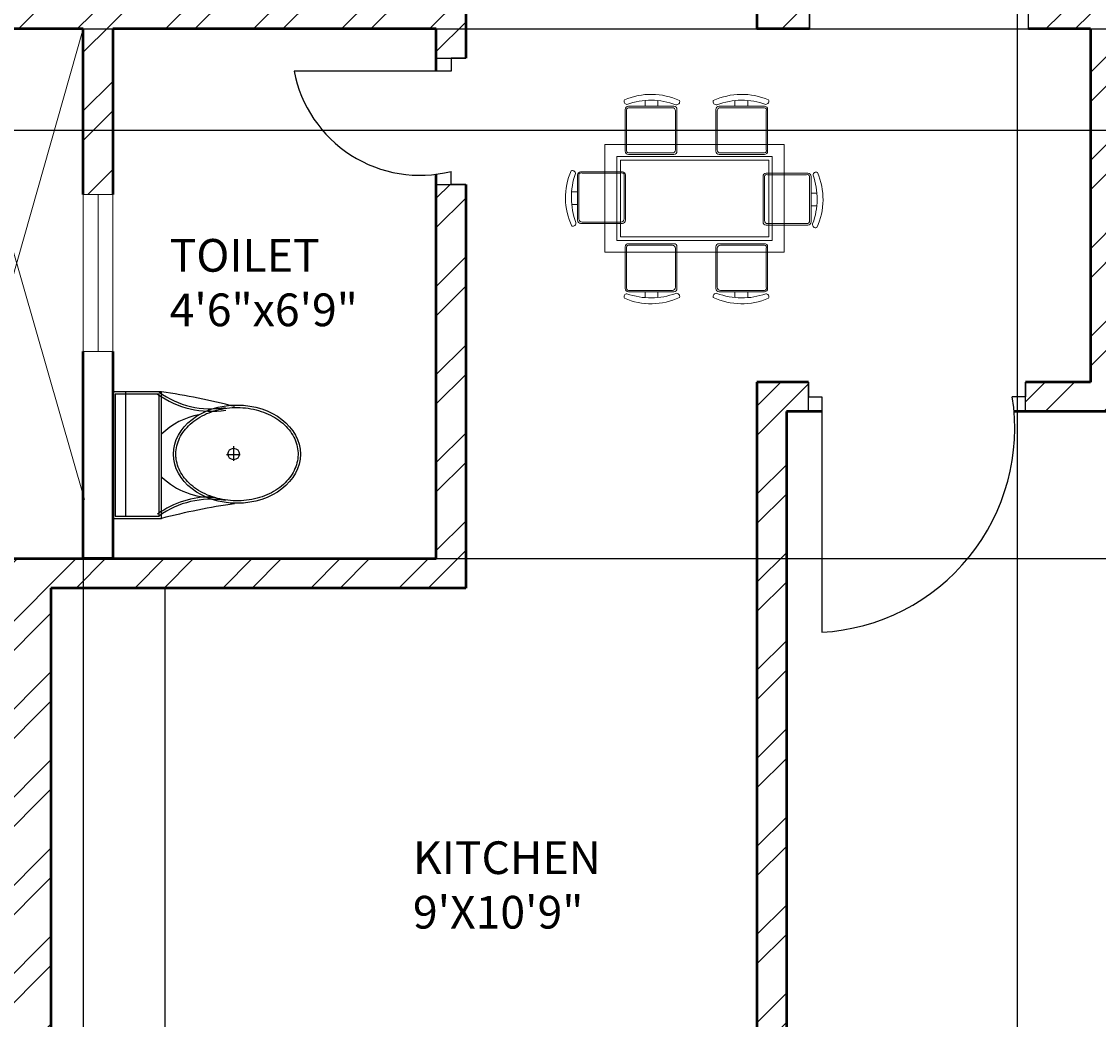
# Model space of a CAD drawing. Units: inches. Extents: x 1980 to 2738, y 1471 to 2568.
# Tile 12 of 22: x 2363 to 2528, y 1722 to 1874. Entities that reach past the tile are written whole.
import ezdxf

# ---------------------------------------------------------------- set-up
doc = ezdxf.new("R2010")
doc.units = ezdxf.units.IN
for name, color, linetype, lineweight in [('A-ANNO-DIMS', 2, 'Continuous', 18), ('A-AREA-IDEN', 7, 'Continuous', 18), ('A-DOOR', 31, 'Continuous', 25), ('A-FLOR-CASE', 8, 'Continuous', 25), ('A-FLOR-FIXT', 8, 'Continuous', 25), ('A-FLOR-OPEN', 8, 'Continuous', 18), ('A-FURN', 8, 'Continuous', 18), ('A-GLAZ', 141, 'Continuous', 18), ('A-WALL', 7, 'Continuous', 50)]:
    doc.layers.add(name, color=color, linetype=linetype, lineweight=lineweight)
doc.layers.add('A-WALL-PATT', color=9, linetype='Continuous', lineweight=13, true_color=0xd19cc7)
doc.styles.get("Standard").update_dxf_attribs({"font": 'arial.ttf'})
doc.dimstyles.get("Standard").update_dxf_attribs({"dimtxt": 0.18, "dimasz": 0.18, "dimexe": 0.18, "dimexo": 0.0625, "dimgap": 0.09, "dimtad": 0, "dimtih": 1, "dimtoh": 1, "dimdec": 4, "dimzin": 0, "dimdsep": 46, "dimtxsty": 'Standard', "dimcen": 0.09, "dimadec": 0, "dimazin": 0, "dimtfac": 1, "dimtdec": 4, "dimtofl": 0, "dimtmove": 0, "dimatfit": 3, "dimfxl": 1, "dimtolj": 1, "dimtzin": 0, "dimarcsym": 0})

# ---------------------------------------------------------------- blocks, each defined once
blk = doc.blocks.new('A$C31115884')
for p, q in [((283.1, 497.7), (223.4, 497.7)), ((257.5, 466.4), (257.5, 523.2)), ((0, 200), (0, 0)), ((520, 200), (0, 200)), ((10, 190), (10, 10)), ((510, 190), (10, 190)), ((510, 10), (510, 190)), ((520, 0), (520, 200)), ((510, 54.5), (0, 54.5)), ((10, 10), (510, 10)), ((0, 0), (520, 0))]:
    blk.add_line(p, q)
blk.add_circle((255.6, 496.4), 23.6)
for centre, radius, start, end in [((2777.7, -204.6), 2807, 165.4549, 171.7133), ((3237, 905), 2807, 188.2867, 194.5451), ((-294.5, 403.3), 364.7, 324.2091, 9.3499), ((-294.5, 403.3), 374.7, 324.2091, 9.3499), ((805.8, 403.3), 364.7, 170.6501, 215.7909), ((139.5, 406.2), 293.5, 315.8436, 2.6563), ((805.8, 403.3), 374.7, 179.2036, 215.7909), ((383.6, 406.2), 293.5, 190.2774, 224.1564)]:
    blk.add_arc(centre, radius, start, end)
blk.add_ellipse((256.2, 509.9), major_axis=(0, -260.7), ratio=0.772727)
blk.add_open_spline([(256.2, 259.2), (263.1, 259.2), (270, 259.7), (287.8, 262.3), (298.7, 265.1), (319.9, 273.1), (330.2, 278.4), (350.1, 291.1), (359.7, 298.7), (377.7, 315.9), (386.2, 325.5), (401.7, 346.6), (408.8, 358.1), (421.3, 382.5), (426.8, 395.5), (435.9, 422.4), (439.5, 436.4), (444.8, 465.1), (446.5, 479.7), (447.9, 509.2), (447.6, 524), (445, 553.3), (442.7, 567.8), (436.3, 596), (432.1, 609.7), (421.9, 636), (416, 648.6), (402.5, 672.1), (395, 683), (378.6, 703), (369.8, 712.1), (351.1, 728), (341.3, 734.8), (320.9, 746.2), (310.4, 750.7), (288.9, 757.3), (278, 759.4), (256, 761), (245, 760.6), (223.1, 757.2), (212.3, 754.3), (191.1, 746.1), (180.8, 740.7), (160.9, 727.8), (151.4, 720.1), (133.5, 702.7), (125.1, 693), (109.6, 671.7), (102.6, 660.2), (90.2, 635.7), (84.9, 622.7), (76, 595.6), (72.4, 581.6), (67.2, 552.9), (65.6, 538.2), (64.4, 508.8), (64.8, 494), (67.5, 464.7), (69.9, 450.2), (76.6, 422), (80.8, 408.3), (91.1, 382.2), (97.2, 369.7), (110.8, 346.3), (118.4, 335.4), (134.8, 315.6), (143.7, 306.7), (162.4, 290.9), (172.3, 284.2), (192.8, 273), (203.3, 268.6), (224.8, 262.2), (235.8, 260.2), (249.9, 259.3), (253, 259.2), (256.2, 259.2)], degree=3, knots=[0, 0, 0, 0, 0.110105, 0.110105, 0.285049, 0.285049, 0.459994, 0.459994, 0.634938, 0.634938, 0.809882, 0.809882, 0.984827, 0.984827, 1.159771, 1.159771, 1.334715, 1.334715, 1.50966, 1.50966, 1.684604, 1.684604, 1.859549, 1.859549, 2.034493, 2.034493, 2.209437, 2.209437, 2.384382, 2.384382, 2.559326, 2.559326, 2.73427, 2.73427, 2.909215, 2.909215, 3.084159, 3.084159, 3.259103, 3.259103, 3.434048, 3.434048, 3.608992, 3.608992, 3.783936, 3.783936, 3.958881, 3.958881, 4.133825, 4.133825, 4.30877, 4.30877, 4.483714, 4.483714, 4.658658, 4.658658, 4.833603, 4.833603, 5.008547, 5.008547, 5.183491, 5.183491, 5.358436, 5.358436, 5.53338, 5.53338, 5.708324, 5.708324, 5.883269, 5.883269, 6.058213, 6.058213, 6.233158, 6.233158, 6.283185, 6.283185, 6.283185, 6.283185])
blk = doc.blocks.new('TABLE-DINING-RECT')
for points in [[(0, 16.47), (27.45, 16.47), (27.45, 0), (0, 0)], [(0, 16.47), (27.45, 16.47), (27.45, 0), (0, 0)], [(1.83, 14.64), (25.62, 14.64), (25.62, 1.83), (1.83, 1.83)], [(1.83, 14.64), (25.62, 14.64), (25.62, 1.83), (1.83, 1.83)], [(2.38, 14.09), (25.07, 14.09), (25.07, 2.38), (2.38, 2.38)], [(2.38, 14.09), (25.07, 14.09), (25.07, 2.38), (2.38, 2.38)]]:
    blk.add_lwpolyline(points, close=True)
blk = doc.blocks.new('WIN-24IN-PARTITION')
for p, q in [((0, 24), (4.5, 24)), ((0, 24), (0, 0)), ((4.5, 24), (2.25, 24)), ((2.25, 24), (2.25, 0)), ((4.5, 24), (4.5, 0)), ((2.25, 0), (0, 0)), ((0, 0), (4.5, 0))]:
    blk.add_line(p, q)
blk = doc.blocks.new('SHAFT-OPENING-MARK')
for p, q in [((20.51, 72), (0, 0)), ((0, 72), (20.71, 0.06))]:
    blk.add_line(p, q)
blk = doc.blocks.new('*D41')
at = {"layer": 'A-ANNO-DIMS', "color": 0, "lineweight": -2, "transparency": 16777216}
for p, q in [((2298.65, 2095.14), (2298.65, 1533.71)), ((2515.4, 2095.14), (2515.4, 1533.71)), ((2298.83, 1533.89), (2406.56, 1533.89)), ((2515.22, 1533.89), (2407.49, 1533.89))]:
    blk.add_line(p, q, dxfattribs=at)
at = {"layer": 'A-ANNO-DIMS', "color": 0, "transparency": 16777216}
for points in [[(2298.83, 1533.92), (2298.83, 1533.86), (2298.65, 1533.89)], [(2515.22, 1533.92), (2515.22, 1533.86), (2515.4, 1533.89)]]:
    blk.add_solid(points, dxfattribs=at)
at = {"layer": 'Defpoints', "color": 0, "transparency": 16777216}
for p in [(2298.65, 2095.21), (2515.4, 2095.21), (2515.4, 1533.89)]:
    blk.add_point(p, dxfattribs=at)
at = {"layer": 'A-ANNO-DIMS', "color": 0, "transparency": 16777216, "insert": (2407.03, 1533.89), "char_height": 0.18, "attachment_point": 5}
blk.add_mtext('\\A1;216.75', dxfattribs=at)
blk = doc.blocks.new('*D57')
at = {"layer": 'A-ANNO-DIMS', "color": 0, "lineweight": -2, "transparency": 16777216}
for p, q in [((2351.81, 1792.14), (2351.81, 1533.71)), ((2372.53, 1792.14), (2372.53, 1533.71)), ((2351.99, 1533.89), (2361.77, 1533.89)), ((2372.35, 1533.89), (2362.56, 1533.89))]:
    blk.add_line(p, q, dxfattribs=at)
at = {"layer": 'A-ANNO-DIMS', "color": 0, "transparency": 16777216}
for points in [[(2351.99, 1533.92), (2351.99, 1533.86), (2351.81, 1533.89)], [(2372.35, 1533.92), (2372.35, 1533.86), (2372.53, 1533.89)]]:
    blk.add_solid(points, dxfattribs=at)
at = {"layer": 'Defpoints', "color": 0, "transparency": 16777216}
for p in [(2351.81, 1792.21), (2372.53, 1792.21), (2372.53, 1533.89)]:
    blk.add_point(p, dxfattribs=at)
at = {"layer": 'A-ANNO-DIMS', "color": 0, "transparency": 16777216, "insert": (2362.17, 1533.89), "char_height": 0.18, "attachment_point": 5}
blk.add_mtext('\\A1;20.72', dxfattribs=at)
blk = doc.blocks.new('*D58')
at = {"layer": 'A-ANNO-DIMS', "color": 0, "lineweight": -2, "transparency": 16777216}
for p, q in [((2372.59, 1873.21), (2689.91, 1873.21)), ((2689.73, 1873.03), (2689.73, 1832.89)), ((2689.73, 1792.39), (2689.73, 1832.52)), ((2372.59, 1792.21), (2689.91, 1792.21))]:
    blk.add_line(p, q, dxfattribs=at)
at = {"layer": 'A-ANNO-DIMS', "color": 0, "transparency": 16777216}
for points in [[(2689.7, 1873.03), (2689.76, 1873.03), (2689.73, 1873.21)], [(2689.7, 1792.39), (2689.76, 1792.39), (2689.73, 1792.21)]]:
    blk.add_solid(points, dxfattribs=at)
at = {"layer": 'Defpoints', "color": 0, "transparency": 16777216}
for p in [(2372.53, 1873.21), (2689.73, 1873.21), (2372.53, 1792.21)]:
    blk.add_point(p, dxfattribs=at)
at = {"layer": 'A-ANNO-DIMS', "color": 0, "transparency": 16777216, "insert": (2689.73, 1832.71), "char_height": 0.18, "attachment_point": 5}
blk.add_mtext('\\A1;81', dxfattribs=at)
blk = doc.blocks.new('*D61')
at = {"layer": 'A-ANNO-DIMS', "color": 0, "lineweight": -2, "transparency": 16777216}
for p, q in [((2114.15, 1873.21), (2689.91, 1873.21)), ((2689.73, 1873.03), (2689.73, 1865.65)), ((2689.73, 1857.91), (2689.73, 1865.29)), ((2114.15, 1857.73), (2689.91, 1857.73))]:
    blk.add_line(p, q, dxfattribs=at)
at = {"layer": 'A-ANNO-DIMS', "color": 0, "transparency": 16777216}
for points in [[(2689.7, 1873.03), (2689.76, 1873.03), (2689.73, 1873.21)], [(2689.7, 1857.91), (2689.76, 1857.91), (2689.73, 1857.73)]]:
    blk.add_solid(points, dxfattribs=at)
at = {"layer": 'Defpoints', "color": 0, "transparency": 16777216}
for p in [(2114.08, 1873.21), (2689.73, 1873.21), (2114.08, 1857.73)]:
    blk.add_point(p, dxfattribs=at)
at = {"layer": 'A-ANNO-DIMS', "color": 0, "transparency": 16777216, "insert": (2689.73, 1865.47), "char_height": 0.18, "attachment_point": 5}
blk.add_mtext('\\A1;15.48', dxfattribs=at)

msp = doc.modelspace()

# ---------------------------------------------------------------- hatches: boundary and pattern name
at = {"layer": 'A-WALL-PATT'}
h = msp.add_hatch(dxfattribs=at)
h.set_pattern_fill('ANSI32', color=256)
h.paths.add_polyline_path([(2257.5661, 2416.2064), (2257.5661, 2420.7064), (2250.5833, 2420.7064), (2250.5833, 2462.7064), (2246.0833, 2462.7064), (2246.0833, 2420.7064), (2237.0791, 2420.7064), (2237.0791, 2411.7064), (2246.0833, 2411.7064), (2246.0833, 2291.7064), (2242.6109, 2291.7064), (2242.6109, 2287.2064), (2246.0833, 2287.2064), (2250.5833, 2287.2064), (2250.5833, 2291.7064), (2250.5833, 2411.7064), (2257.5661, 2411.7064)])
h.paths.add_polyline_path([(2387.0396, 2416.2064), (2387.0396, 2420.7064), (2367.5833, 2420.7064), (2367.5833, 2462.7064), (2358.5833, 2462.7064), (2358.5833, 2420.7064), (2329.3087, 2420.7064), (2329.3087, 2411.7064), (2358.5833, 2411.7064), (2358.5833, 2321.7275), (2358.5833, 2309.7064), (2347.3089, 2309.7064), (2293.3089, 2309.7064), (2293.3089, 2259.0771), (2297.8089, 2259.0771), (2297.8089, 2305.2064), (2347.3089, 2305.2064), (2347.3089, 2284.7412), (2351.8089, 2284.7412), (2351.8089, 2305.2064), (2372.3188, 2305.2064), (2372.3761, 2284.3899), (2377.0295, 2284.3899), (2377.0295, 2299.3058), (2377.0295, 2305.2064), (2426.5295, 2305.2064), (2426.5295, 2257.5573), (2431.0295, 2257.5573), (2431.0295, 2309.7064), (2377.0295, 2309.7064), (2367.5833, 2309.7064), (2367.5833, 2321.7275), (2367.5833, 2411.7064), (2387.0396, 2411.7064)])
h.paths.add_polyline_path([(2448.5267, 2416.2064), (2448.5267, 2420.7064), (2423.0396, 2420.7064), (2423.0396, 2411.7064), (2448.5267, 2411.7064)])
h.paths.add_polyline_path([(2130.9128, 2416.2064), (2130.9128, 2420.7064), (2105.0833, 2420.7064), (2105.0833, 2386.6942), (2114.0833, 2386.6942), (2114.0833, 2411.7064), (2130.9128, 2411.7064)])
h.paths.add_polyline_path([(2212.9478, 2420.7064), (2190.9128, 2420.7064), (2190.9128, 2411.7064), (2212.9478, 2411.7064), (2212.9478, 2416.2064)])
h.paths.add_polyline_path([(2114.0833, 2326.6942), (2105.0833, 2326.6942), (2105.0833, 2291.7064), (2081.0833, 2291.7064), (2081.0833, 2287.2064), (2105.0833, 2287.2064), (2105.0833, 2276.1935), (2114.0833, 2276.1935), (2114.0833, 2287.2064), (2166.3825, 2287.2064), (2166.3825, 2289.4564), (2166.3825, 2291.7064), (2114.0833, 2291.7064)])
h.paths.add_polyline_path([(2114.0833, 2252.1935), (2105.0833, 2252.1935), (2105.0833, 2233.2064), (2081.0833, 2233.2064), (2081.0833, 2228.7064), (2105.0833, 2228.7064), (2105.0833, 2213.4478), (2114.0833, 2213.4478), (2114.0833, 2228.7064), (2195.0833, 2228.7064), (2199.5833, 2228.7064), (2208.4455, 2228.7064), (2208.4455, 2230.9564), (2208.4455, 2233.2064), (2199.5833, 2233.2064), (2199.5833, 2287.2064), (2206.8904, 2287.2064), (2206.8904, 2289.4564), (2206.8904, 2291.7064), (2189.446, 2291.7064), (2189.446, 2289.4564), (2189.446, 2287.2064), (2195.0833, 2287.2064), (2195.0833, 2233.2064), (2114.0833, 2233.2064)])
h.paths.add_polyline_path([(2114.0833, 2153.4478), (2109.5833, 2153.4478), (2105.0833, 2153.4478), (2105.0833, 2135.2374), (2114.0833, 2135.2374)], flags=17)
h.paths.add_polyline_path([(2135.9619, 2095.4081), (2140.1805, 2095.4081), (2140.1805, 2104.2064), (2114.0833, 2104.2064), (2114.0833, 2110.3997), (2109.5833, 2110.3997), (2105.0833, 2110.3997), (2105.0833, 2104.2064), (2081.0833, 2104.2064), (2081.0833, 2099.7064), (2105.0833, 2099.7064), (2127.5416, 2099.8532), (2127.5416, 2056.9393), (2136.2133, 2056.9393)], flags=17)
h.paths.add_polyline_path([(2255.4895, 2104.2064), (2250.5833, 2104.2064), (2250.5833, 2233.2064), (2246.0833, 2233.2064), (2242.4941, 2233.2064), (2242.4941, 2228.7064), (2246.0833, 2228.7064), (2246.0833, 2104.2064), (2163.6825, 2104.2064), (2163.6825, 2099.8072), (2163.6825, 2095.4081), (2191.4325, 2095.4081), (2191.4325, 2011.2064), (2186.0833, 2011.2064), (2136.5143, 2010.8824), (2136.3702, 2032.9403), (2131.9559, 2032.9115), (2127.5416, 2032.8826), (2127.5416, 2006.7064), (2105.0833, 2006.7064), (2081.0833, 2006.7064), (2081.0833, 2002.2064), (2105.0833, 2002.2064), (2105.0833, 1995.9329), (2114.0833, 1995.9329), (2114.0833, 2002.2064), (2246.0833, 2002.2064), (2246.0833, 1877.7064), (2242.1358, 1877.7064), (2242.1358, 1873.2064), (2250.5833, 1873.2064), (2250.5833, 2002.2064), (2255.3335, 2002.2064), (2255.3335, 2011.2064), (2195.9325, 2011.2064), (2195.9325, 2095.2064), (2255.4895, 2095.2064), (2255.4895, 2099.5471)])
h.paths.add_polyline_path([(2199.5833, 1873.2064), (2209.827, 1873.2064), (2209.827, 1875.4564), (2209.827, 1877.7064), (2114.0833, 1877.7064), (2114.0833, 1890.0968), (2105.0833, 1890.0968), (2105.0833, 1877.7064), (2081.0833, 1877.7064), (2081.0833, 1873.2064), (2105.0833, 1873.2064), (2105.0833, 1857.7279), (2114.0833, 1857.7279), (2114.0833, 1873.2064), (2195.0833, 1873.2064), (2195.0833, 1819.2064), (2190.298, 1819.2064), (2190.298, 1814.7064), (2209.8976, 1814.7064), (2209.8976, 1816.9564), (2209.8976, 1819.2064), (2199.5833, 1819.2064)])
h.paths.add_polyline_path([(2114.0833, 1814.7064), (2166.2538, 1814.7064), (2166.2538, 1816.9564), (2166.2538, 1819.2064), (2114.0833, 1819.2064), (2114.0833, 1833.7279), (2109.5833, 1833.7279), (2105.0833, 1833.7279), (2105.0833, 1819.2064), (2081.0833, 1819.2064), (2081.0833, 1814.7064), (2105.0833, 1814.7064), (2105.0833, 1782.5516), (2114.0833, 1782.5516)])
h.paths.add_polyline_path([(2114.0833, 1722.5516), (2109.5833, 1722.5516), (2105.0833, 1722.5516), (2105.0833, 1685.7064), (2124.5104, 1685.7064), (2124.5104, 1690.2064), (2124.5104, 1694.7064), (2114.0833, 1694.7064)])
h.paths.add_polyline_path([(2218.8787, 1694.7064), (2184.5104, 1694.7064), (2184.5104, 1685.7064), (2218.8787, 1685.7064), (2218.8787, 1690.2064)])
h.paths.add_polyline_path([(2250.5833, 1819.2064), (2242.6431, 1819.2064), (2242.6431, 1816.9564), (2242.6431, 1814.7064), (2246.0833, 1814.7064), (2246.0833, 1694.7064), (2240.4035, 1694.7064), (2240.4035, 1690.2064), (2240.4035, 1685.7064), (2246.0833, 1685.7064), (2246.0833, 1643.7064), (2250.5833, 1643.7064), (2250.5833, 1685.7064), (2255.9859, 1685.7064), (2255.9859, 1690.2064), (2255.9859, 1694.7064), (2250.5833, 1694.7064)])
h.paths.add_polyline_path([(2297.4764, 1694.7064), (2279.3934, 1694.7064), (2279.3934, 1690.2064), (2279.3934, 1685.7064), (2297.4764, 1685.7064), (2297.4764, 1690.2064)])
h.paths.add_polyline_path([(2377.1596, 1694.7064), (2367.5833, 1694.7064), (2367.5833, 1787.7064), (2431.0295, 1787.7064), (2431.0295, 1792.2064), (2431.0295, 1849.4149), (2428.7795, 1849.4149), (2426.5295, 1849.4149), (2426.5295, 1792.2064), (2421.5833, 1792.2064), (2367.5833, 1792.2064), (2297.8089, 1792.2064), (2297.8089, 1850.2946), (2295.5589, 1850.2946), (2293.3089, 1850.2946), (2293.3089, 1792.2064), (2293.3089, 1787.7064), (2297.8089, 1787.7064), (2358.5833, 1787.7064), (2358.5833, 1694.7064), (2333.4764, 1694.7064), (2333.4764, 1685.7064), (2358.5833, 1685.7064), (2358.5833, 1643.7064), (2367.5833, 1643.7064), (2367.5833, 1685.7064), (2377.1596, 1685.7064)])
h.paths.add_polyline_path([(2442.4912, 1694.7064), (2413.1596, 1694.7064), (2413.1596, 1685.7064), (2442.4912, 1685.7064)])
h.paths.add_polyline_path([(2480.0833, 1814.7064), (2483.4816, 1814.7064), (2483.4816, 1817.9384), (2483.4816, 1819.2064), (2475.5833, 1819.2064), (2475.5833, 1694.7064), (2470.7283, 1694.7064), (2470.7283, 1685.7064), (2475.5833, 1685.7064), (2475.5833, 1643.7064), (2480.0833, 1643.7064), (2480.0833, 1685.7064), (2486.3293, 1685.7064), (2486.3293, 1690.2064), (2486.3293, 1694.7064), (2480.0833, 1694.7064)])
h.paths.add_polyline_path([(2621.0833, 1721.7349), (2612.0833, 1721.7349), (2612.0833, 1694.7064), (2586.1453, 1694.7064), (2586.1453, 1685.7064), (2621.0833, 1685.7064)])
h.paths.add_polyline_path([(2526.1453, 1690.2064), (2526.1453, 1694.7064), (2511.584, 1694.7064), (2511.584, 1690.2064), (2511.584, 1685.7064), (2526.1453, 1685.7064)])
h.paths.add_polyline_path([(2645.0833, 1819.2064), (2621.0833, 1819.2064), (2621.0833, 1835.8527), (2616.5833, 1835.8527), (2612.0833, 1835.8527), (2612.0833, 1819.2064), (2560.2541, 1819.2064), (2560.2541, 1814.7064), (2612.0833, 1814.7064), (2612.0833, 1781.7349), (2621.0833, 1781.7349), (2621.0833, 1814.7064), (2645.0833, 1814.7064)])
h.paths.add_polyline_path([(2645.0833, 1877.7064), (2621.0833, 1877.7064), (2621.0833, 1886.4375), (2612.0833, 1886.4375), (2612.0833, 1877.7064), (2517.1032, 1877.7064), (2517.1032, 1875.4564), (2517.1032, 1873.2064), (2526.5833, 1873.2064), (2526.5833, 1819.2064), (2516.6454, 1819.2064), (2516.6454, 1816.9564), (2516.6454, 1814.7064), (2536.4445, 1814.7064), (2536.4445, 1816.9564), (2536.4445, 1819.2064), (2531.0833, 1819.2064), (2531.0833, 1873.2064), (2612.0833, 1873.2064), (2612.0833, 1859.8527), (2621.0833, 1859.8527), (2621.0833, 1873.2064), (2645.0833, 1873.2064)])
h.paths.add_polyline_path([(2645.0833, 2006.7064), (2621.0833, 2006.7064), (2588.5085, 2006.7064), (2588.5085, 2052.9125), (2579.9045, 2052.9125), (2579.9045, 2011.2064), (2519.9045, 2011.2064), (2519.9045, 2095.2064), (2553.1204, 2095.2064), (2553.1204, 2104.2064), (2480.0833, 2104.2064), (2480.0833, 2228.7064), (2484.3832, 2228.7064), (2484.3832, 2230.9564), (2484.3832, 2233.2064), (2475.5833, 2233.2064), (2475.5833, 2104.2064), (2463.1308, 2104.2064), (2463.1308, 2095.2064), (2501.2463, 2095.2064), (2510.9045, 2095.2064), (2515.4045, 2095.2064), (2515.4045, 2011.2064), (2510.9045, 2011.2064), (2501.2463, 2011.2064), (2462.5957, 2011.2064), (2462.5957, 2002.2064), (2475.5833, 2002.2064), (2475.5833, 1873.2064), (2483.6146, 1873.2064), (2483.6146, 1875.4564), (2483.6146, 1877.7064), (2480.0833, 1877.7064), (2480.0833, 2002.2064), (2612.0833, 2002.2064), (2612.0833, 1996.309), (2621.0833, 1996.309), (2621.0833, 2002.2064), (2645.0833, 2002.2064)])
h.paths.add_polyline_path([(2588.5085, 2099.7277), (2621.0833, 2099.7277), (2645.0833, 2099.7064), (2645.0833, 2104.2064), (2621.0833, 2104.2064), (2621.0833, 2109.0038), (2616.5833, 2109.0038), (2612.0833, 2109.0038), (2612.0833, 2104.2064), (2575.0621, 2104.2064), (2575.0621, 2099.7064), (2575.0621, 2095.2064), (2579.9045, 2095.2064), (2579.9045, 2076.9125), (2588.5085, 2076.9125)], flags=17)
h.paths.add_polyline_path([(2367.5833, 2002.2064), (2373.7228, 2002.2064), (2373.7228, 2006.7064), (2373.7228, 2011.2064), (2350.7889, 2011.2064), (2350.7889, 2006.7064), (2350.7889, 2002.2064), (2358.5833, 2002.2064), (2358.5833, 1877.7064), (2293.3089, 1877.7064), (2293.3089, 1870.4987), (2297.8089, 1870.4987), (2297.8089, 1873.2064), (2347.3089, 1873.2064), (2347.3089, 1847.2208), (2351.8089, 1847.2208), (2351.8089, 1873.2064), (2372.5295, 1873.2064), (2372.5295, 1847.8619), (2377.0295, 1847.8619), (2377.0295, 1873.2064), (2426.5295, 1873.2064), (2426.5295, 1868.7339), (2431.0295, 1868.7339), (2431.0295, 1877.7064), (2367.5833, 1877.7064)])
h.paths.add_polyline_path([(2531.0833, 2287.2064), (2534.2285, 2287.2064), (2534.2285, 2291.7064), (2516.7886, 2291.7064), (2516.7886, 2287.2064), (2526.5833, 2287.2064), (2526.5833, 2233.2064), (2517.9112, 2233.2064), (2517.9112, 2230.9564), (2517.9112, 2228.7064), (2526.5833, 2228.7064), (2531.0833, 2228.7064), (2612.0833, 2228.7064), (2612.0833, 2206.8504), (2621.0833, 2206.8504), (2621.0833, 2228.7064), (2645.0833, 2228.7064), (2645.0833, 2233.2064), (2621.0833, 2233.2064), (2621.0833, 2241.8536), (2616.5833, 2241.8536), (2612.0833, 2241.8536), (2612.0833, 2233.2064), (2531.0833, 2233.2064)])
h.paths.add_polyline_path([(2645.0833, 2291.7064), (2621.0833, 2291.7064), (2621.0833, 2323.0138), (2616.5833, 2323.0138), (2612.0833, 2323.0138), (2612.0833, 2291.7064), (2559.6852, 2291.7064), (2559.6852, 2289.4564), (2559.6852, 2287.2064), (2612.0833, 2287.2064), (2612.0833, 2265.8536), (2621.0833, 2265.8536), (2621.0833, 2287.2064), (2645.0833, 2287.2064)])
h.paths.add_polyline_path([(2621.0833, 2420.7064), (2582.8189, 2420.7064), (2582.8189, 2411.7064), (2612.0833, 2411.7064), (2612.0833, 2383.0138), (2621.0833, 2383.0138)])
h.paths.add_polyline_path([(2480.0833, 2411.7064), (2485.7342, 2411.7064), (2485.7342, 2416.2064), (2485.7342, 2420.7064), (2480.0833, 2420.7064), (2480.0833, 2462.7064), (2475.5833, 2462.7064), (2475.5833, 2420.7064), (2469.4083, 2420.7064), (2469.4083, 2411.7064), (2475.5833, 2411.7064), (2475.5833, 2291.7064), (2475.5833, 2287.2064), (2482.9195, 2287.2064), (2482.9195, 2289.4564), (2482.9195, 2291.7064), (2480.0833, 2291.7064)])
h.paths.add_polyline_path([(2367.5833, 2228.7064), (2431.0295, 2228.7064), (2431.0295, 2233.2064), (2431.0295, 2237.4203), (2428.7795, 2237.4203), (2426.5295, 2237.4203), (2426.5295, 2233.2064), (2377.0295, 2233.2064), (2377.0295, 2260.3837), (2372.4423, 2260.3837), (2372.517, 2233.2635), (2351.8089, 2233.2064), (2351.8089, 2260.7412), (2347.3089, 2260.7412), (2347.3089, 2233.2064), (2297.8089, 2233.2064), (2297.8089, 2236.9324), (2293.3089, 2236.9324), (2293.3089, 2228.7064), (2358.5833, 2228.7064), (2358.5833, 2104.2064), (2353.3665, 2104.2064), (2353.3665, 2095.2064), (2373.8869, 2095.2064), (2373.8869, 2099.7064), (2373.8869, 2104.2064), (2367.5833, 2104.2064)])
h.paths.add_polyline_path([(2321.2323, 2104.2064), (2303.4895, 2104.2064), (2303.4895, 2095.2064), (2321.2323, 2095.2064), (2321.2323, 2099.7064)], flags=0)
h.paths.add_polyline_path([(2415.1308, 2099.7064), (2415.1308, 2104.2064), (2404.81, 2104.2064), (2404.81, 2095.2064), (2415.1308, 2095.2064)], flags=17)
h.paths.add_polyline_path([(2318.6336, 2011.2064), (2303.3335, 2011.2064), (2303.3335, 2002.2064), (2318.6336, 2002.2064)], flags=0)
h.paths.add_polyline_path([(2414.5957, 2011.2064), (2406.2461, 2011.2064), (2406.2461, 2006.7064), (2406.2461, 2002.2064), (2414.5957, 2002.2064)], flags=17)

# ---------------------------------------------------------------- linework, layer by layer
at = {"layer": 'A-DOOR'}
for p, q in [((2483.6146, 1877.7064), (2483.6146, 1873.2064)), ((2517.1032, 1873.2064), (2517.1032, 1877.7064)), ((2483.6146, 1873.2064), (2483.6146, 1875.4564)), ((2426.5295, 1868.7339), (2431.0295, 1868.7339)), ((2431.0295, 1868.7339), (2428.7795, 1868.7339)), ((2428.7795, 1868.7339), (2428.7795, 1868.7339)), ((2428.7795, 1868.7339), (2428.7795, 1866.7339)), ((2428.7795, 1866.7339), (2404.7795, 1866.7339)), ((2428.7795, 1849.4149), (2428.7795, 1851.4149)), ((2426.5295, 1849.4149), (2431.0295, 1849.4149)), ((2431.0295, 1849.4149), (2428.7795, 1849.4149)), ((2483.4816, 1817.9384), (2483.4816, 1819.2064)), ((2483.4816, 1819.2064), (2483.4816, 1816.9444)), ((2516.6454, 1814.7064), (2516.6454, 1819.2064)), ((2516.6454, 1819.2064), (2516.6454, 1816.9564)), ((2483.4816, 1814.7064), (2483.4816, 1817.9384)), ((2483.4816, 1816.9444), (2485.4816, 1816.9444)), ((2485.4816, 1816.9444), (2485.4816, 1780.9444)), ((2516.6454, 1816.9564), (2514.6454, 1816.9564))]:
    msp.add_line(p, q, dxfattribs=at)
for centre, radius, start, end in [((2424.0189, 1870.4161), 19.5886, 190.83485, 284.065556), ((2483.7368, 1812.1723), 31.2767, 273.198076, 8.798569)]:
    msp.add_arc(centre, radius, start, end, dxfattribs=at)
at = {"layer": 'A-FLOR-CASE'}
msp.add_line((2384.9917, 1787.7064), (2384.9917, 1711.1804), dxfattribs=at)
at = {"layer": 'A-FURN'}
for points in [[(2455.6982, 1861.6711, -0.17580919), (2463.1736, 1861.6144, 0.57839206), (2463.7399, 1862.2372, 0.21452438), (2455.3018, 1862.3504, 0.55201397), (2455.6982, 1861.6711, -0.06507904)], [(2455.6982, 1861.6708, -0.17580919), (2463.1736, 1861.6142, 0.57839206), (2463.74, 1862.2369, 0.21452438), (2455.3018, 1862.3501, 0.55201397), (2455.6982, 1861.6708, -0.06507904)], [(2469.467, 1861.6144, -0.57839206), (2468.9006, 1862.2372, -0.21452438), (2477.3388, 1862.3504, -0.55201397), (2476.9424, 1861.6711, 0.1758092), (2469.467, 1861.6144)], [(2469.467, 1861.6142, -0.57839206), (2468.9007, 1862.2369, -0.21452438), (2477.3388, 1862.3501, -0.55201397), (2476.9424, 1861.6708, 0.1758092), (2469.467, 1861.6142)], [(2460.4188, 1861.371), (2460.4188, 1862.2487, -0.06475861)], [(2460.4188, 1861.3707), (2460.4188, 1862.2484, -0.06475861)], [(2472.2218, 1861.371), (2472.2218, 1862.2487, 0.06475861)], [(2472.2218, 1861.3707), (2472.2218, 1862.2484, 0.06475861)], [(2462.8565, 1861.371), (2455.9165, 1861.371, 0.41421356), (2455.431, 1860.8855), (2455.431, 1854.5044, 0.41421356), (2455.9165, 1854.0188), (2462.8565, 1854.0188, 0.41421356), (2463.342, 1854.5044), (2463.342, 1860.8855, 0.41421356), (2462.8565, 1861.371)], [(2462.8565, 1861.3707), (2455.9165, 1861.3707, 0.41421356), (2455.431, 1860.8852), (2455.431, 1854.5041, 0.41421356), (2455.9165, 1854.0185), (2462.8565, 1854.0185, 0.41421356), (2463.342, 1854.5041), (2463.342, 1860.8852, 0.41421356), (2462.8565, 1861.3707)], [(2476.7241, 1861.371, -0.41421356), (2477.2096, 1860.8855), (2477.2096, 1854.5044, -0.41421356), (2476.7241, 1854.0188), (2469.7841, 1854.0188, -0.41421356), (2469.2986, 1854.5044), (2469.2986, 1860.8855, -0.41421356), (2469.7841, 1861.371), (2476.7241, 1861.371)], [(2476.7241, 1861.3707, -0.41421356), (2477.2096, 1860.8852), (2477.2096, 1854.5041, -0.41421356), (2476.7241, 1854.0185), (2469.7841, 1854.0185, -0.41421356), (2469.2986, 1854.5041), (2469.2986, 1860.8852, -0.41421356), (2469.7841, 1861.3707), (2476.7241, 1861.3707)], [(2447.8774, 1843.619, -0.57839206), (2447.2547, 1843.0527, -0.21452438), (2447.1415, 1851.4909, -0.55201397), (2447.8208, 1851.0944, 0.17580937), (2447.8774, 1843.619)], [(2447.8775, 1843.6187, -0.57839206), (2447.2547, 1843.0524, -0.21452438), (2447.1415, 1851.4906, -0.55201397), (2447.8208, 1851.0942, 0.17580937), (2447.8775, 1843.6187)], [(2448.1209, 1850.8761, -0.41421356), (2448.6064, 1851.3616), (2454.9875, 1851.3616, -0.41421356), (2455.4731, 1850.8761), (2455.4731, 1843.9362, -0.41421356), (2454.9875, 1843.4506), (2448.6064, 1843.4506, -0.41421356), (2448.1209, 1843.9362), (2448.1209, 1850.8761)], [(2448.1209, 1850.8758, -0.41421356), (2448.6064, 1851.3613), (2454.9875, 1851.3613, -0.41421356), (2455.4731, 1850.8758), (2455.4731, 1843.9359, -0.41421356), (2454.9875, 1843.4503), (2448.6064, 1843.4503, -0.41421356), (2448.1209, 1843.9359), (2448.1209, 1850.8758)], [(2483.8583, 1850.6384, 0.41421356), (2483.3728, 1851.1239), (2476.9916, 1851.1239, 0.41421356), (2476.5061, 1850.6384), (2476.5061, 1843.6985, 0.41421356), (2476.9916, 1843.213), (2483.3728, 1843.213, 0.41421356), (2483.8583, 1843.6985), (2483.8583, 1850.6384)], [(2483.8583, 1850.6381, 0.41421356), (2483.3728, 1851.1237), (2476.9917, 1851.1237, 0.41421356), (2476.5061, 1850.6381), (2476.5061, 1843.6982, 0.41421356), (2476.9917, 1843.2127), (2483.3728, 1843.2127, 0.41421356), (2483.8583, 1843.6982), (2483.8583, 1850.6381)], [(2484.1583, 1850.8568, -0.17580919), (2484.1017, 1843.3813, 0.57839206), (2484.7244, 1842.815, 0.21452438), (2484.8377, 1851.2532, 0.55201397), (2484.1583, 1850.8568, -0.06507904)], [(2484.1584, 1850.8565, -0.17580919), (2484.1018, 1843.381, 0.57839206), (2484.7245, 1842.8147, 0.21452438), (2484.8377, 1851.2529, 0.55201397), (2484.1584, 1850.8565, -0.06507904)], [(2448.1209, 1846.3738), (2447.2432, 1846.3738, 0.06475861)], [(2448.1209, 1846.3735), (2447.2432, 1846.3735, 0.06475861)], [(2483.8583, 1846.1361), (2484.736, 1846.1361, -0.06475861)], [(2483.8583, 1846.1358), (2484.736, 1846.1358, -0.06475861)], [(2462.8565, 1833.0053), (2455.9165, 1833.0053, -0.41421356), (2455.431, 1833.4908), (2455.431, 1839.8719, -0.41421356), (2455.9165, 1840.3575), (2462.8565, 1840.3575, -0.41421356), (2463.342, 1839.8719), (2463.342, 1833.4908, -0.41421356), (2462.8565, 1833.0053)], [(2462.8565, 1833.005), (2455.9165, 1833.005, -0.41421356), (2455.431, 1833.4905), (2455.431, 1839.8717, -0.41421356), (2455.9165, 1840.3572), (2462.8565, 1840.3572, -0.41421356), (2463.342, 1839.8717), (2463.342, 1833.4905, -0.41421356), (2462.8565, 1833.005)], [(2476.7241, 1833.0053, 0.41421356), (2477.2096, 1833.4908), (2477.2096, 1839.8719, 0.41421356), (2476.7241, 1840.3575), (2469.7841, 1840.3575, 0.41421356), (2469.2986, 1839.8719), (2469.2986, 1833.4908, 0.41421356), (2469.7841, 1833.0053), (2476.7241, 1833.0053)], [(2476.7241, 1833.005, 0.41421356), (2477.2096, 1833.4905), (2477.2096, 1839.8717, 0.41421356), (2476.7241, 1840.3572), (2469.7841, 1840.3572, 0.41421356), (2469.2986, 1839.8717), (2469.2986, 1833.4905, 0.41421356), (2469.7841, 1833.005), (2476.7241, 1833.005)], [(2463.1736, 1832.7619, -0.57839206), (2463.7399, 1832.1391, -0.21452438), (2455.3018, 1832.0259, -0.55201397), (2455.6982, 1832.7052, 0.17580929), (2463.1736, 1832.7619)], [(2463.1736, 1832.7616, -0.57839206), (2463.74, 1832.1389, -0.21452438), (2455.3018, 1832.0256, -0.55201397), (2455.6982, 1832.705, 0.17580929), (2463.1736, 1832.7616)], [(2460.4188, 1833.0053), (2460.4188, 1832.1276, 0.06475861)], [(2460.4188, 1833.005), (2460.4188, 1832.1273, 0.06475861)], [(2476.9424, 1832.7052, -0.17580928), (2469.467, 1832.7619, 0.57839206), (2468.9006, 1832.1391, 0.21452438), (2477.3388, 1832.0259, 0.55201397), (2476.9424, 1832.7052, -0.06507904)], [(2476.9424, 1832.705, -0.17580928), (2469.467, 1832.7616, 0.57839206), (2468.9007, 1832.1389, 0.21452438), (2477.3388, 1832.0256, 0.55201397), (2476.9424, 1832.705, -0.06507904)], [(2472.2218, 1833.0053), (2472.2218, 1832.1276, -0.06475861)], [(2472.2218, 1833.005), (2472.2218, 1832.1273, -0.06475861)]]:
    msp.add_lwpolyline(points, format="xyb", dxfattribs=at)
for points in [[(2458.4762, 1862.2647), (2458.4762, 1861.371)], [(2458.4762, 1862.2644), (2458.4762, 1861.3707)], [(2474.1644, 1862.2647), (2474.1644, 1861.371)], [(2474.1644, 1862.2644), (2474.1644, 1861.3707)], [(2447.2272, 1848.3164), (2448.1209, 1848.3164)], [(2447.2272, 1848.3161), (2448.1209, 1848.3161)], [(2484.752, 1848.0787), (2483.8583, 1848.0787)], [(2484.752, 1848.0784), (2483.8583, 1848.0784)], [(2458.4762, 1832.1116), (2458.4762, 1833.0053)], [(2458.4762, 1832.1113), (2458.4762, 1833.005)], [(2474.1644, 1832.1116), (2474.1644, 1833.0053)], [(2474.1644, 1832.1113), (2474.1644, 1833.005)]]:
    msp.add_lwpolyline(points, dxfattribs=at)
for points in [[(2455.9195, 1861.1523), (2462.6377, 1861.1523, -0.41421356), (2463.1233, 1860.6668), (2463.1233, 1854.7231, -0.41421356), (2462.6377, 1854.2376), (2455.9195, 1854.2376, -0.51206948), (2455.6497, 1854.7231), (2455.6497, 1860.6668, -0.51206948)], [(2455.9195, 1861.152), (2462.6377, 1861.152, -0.41421356), (2463.1233, 1860.6665), (2463.1233, 1854.7228, -0.41421356), (2462.6377, 1854.2373), (2455.9195, 1854.2373, -0.51206948), (2455.6497, 1854.7228), (2455.6497, 1860.6665, -0.51206948)], [(2476.7211, 1861.1523), (2470.0029, 1861.1523, 0.41421356), (2469.5173, 1860.6668), (2469.5173, 1854.7231, 0.41421356), (2470.0029, 1854.2376), (2476.7211, 1854.2376, 0.51206948), (2476.9909, 1854.7231), (2476.9909, 1860.6668, 0.51206948)], [(2476.7211, 1861.152), (2470.0029, 1861.152, 0.41421356), (2469.5173, 1860.6665), (2469.5173, 1854.7228, 0.41421356), (2470.0029, 1854.2373), (2476.7211, 1854.2373, 0.51206948), (2476.9909, 1854.7228), (2476.9909, 1860.6665, 0.51206948)], [(2448.3396, 1850.8732), (2448.3396, 1844.1549, 0.41421356), (2448.8251, 1843.6694), (2454.7688, 1843.6694, 0.41421356), (2455.2543, 1844.1549), (2455.2543, 1850.8732, 0.51206948), (2454.7688, 1851.1429), (2448.8251, 1851.1429, 0.51206948)], [(2448.3396, 1850.8729), (2448.3396, 1844.1546, 0.41421356), (2448.8251, 1843.6691), (2454.7688, 1843.6691, 0.41421356), (2455.2543, 1844.1546), (2455.2543, 1850.8729, 0.51206948), (2454.7688, 1851.1426), (2448.8251, 1851.1426, 0.51206948)], [(2483.6396, 1850.6355), (2483.6396, 1843.9172, -0.41421356), (2483.1541, 1843.4317), (2477.2104, 1843.4317, -0.41421356), (2476.7249, 1843.9172), (2476.7249, 1850.6355, -0.51206948), (2477.2104, 1850.9052), (2483.1541, 1850.9052, -0.51206948)], [(2483.6396, 1850.6352), (2483.6396, 1843.9169, -0.41421356), (2483.1541, 1843.4314), (2477.2104, 1843.4314, -0.41421356), (2476.7249, 1843.9169), (2476.7249, 1850.6352, -0.51206948), (2477.2104, 1850.9049), (2483.1541, 1850.9049, -0.51206948)], [(2455.9195, 1833.224), (2462.6377, 1833.224, 0.41421356), (2463.1233, 1833.7095), (2463.1233, 1839.6532, 0.41421356), (2462.6377, 1840.1387), (2455.9195, 1840.1387, 0.51206948), (2455.6497, 1839.6532), (2455.6497, 1833.7095, 0.51206948)], [(2455.9195, 1833.2237), (2462.6377, 1833.2237, 0.41421356), (2463.1233, 1833.7092), (2463.1233, 1839.6529, 0.41421356), (2462.6377, 1840.1385), (2455.9195, 1840.1385, 0.51206948), (2455.6497, 1839.6529), (2455.6497, 1833.7092, 0.51206948)], [(2476.7211, 1833.224), (2470.0029, 1833.224, -0.41421356), (2469.5173, 1833.7095), (2469.5173, 1839.6532, -0.41421356), (2470.0029, 1840.1387), (2476.7211, 1840.1387, -0.51206948), (2476.9909, 1839.6532), (2476.9909, 1833.7095, -0.51206948)], [(2476.7211, 1833.2237), (2470.0029, 1833.2237, -0.41421356), (2469.5173, 1833.7092), (2469.5173, 1839.6529, -0.41421356), (2470.0029, 1840.1385), (2476.7211, 1840.1385, -0.51206948), (2476.9909, 1839.6529), (2476.9909, 1833.7092, -0.51206948)]]:
    msp.add_lwpolyline(points, format="xyb", close=True, dxfattribs=at)
at = {"layer": 'A-GLAZ'}
msp.add_line((2374.7795, 1847.8619), (2374.7795, 1847.8619), dxfattribs=at)
at = {"layer": 'A-WALL'}
for p, q in [((2475.5833, 2002.2064), (2475.5833, 1873.2064)), ((2431.0295, 1877.7064), (2431.0295, 1868.7339)), ((2372.5295, 1873.2064), (2351.8089, 1873.2064)), ((2372.5295, 1847.8619), (2372.5295, 1873.2064)), ((2426.5295, 1873.2064), (2377.0295, 1873.2064)), ((2377.0295, 1873.2064), (2377.0295, 1847.8619)), ((2426.5295, 1866.7339), (2426.5295, 1873.2064)), ((2483.6146, 1873.2064), (2475.5833, 1873.2064)), ((2526.5833, 1873.2064), (2517.1032, 1873.2064)), ((2526.5833, 1873.2064), (2526.5833, 1819.2064)), ((2426.5295, 1792.2064), (2426.5295, 1850.9891)), ((2431.0295, 1849.4149), (2431.0295, 1792.2064)), ((2372.5295, 1792.2064), (2372.5295, 1823.8619)), ((2377.0295, 1823.8619), (2377.0295, 1792.2064)), ((2475.5833, 1819.2064), (2475.5833, 1694.7064)), ((2483.4816, 1819.2064), (2475.5833, 1819.2064)), ((2526.5833, 1819.2064), (2516.6454, 1819.2064)), ((2480.0833, 1814.7064), (2480.0833, 1694.7064)), ((2485.4816, 1814.7064), (2480.0833, 1814.7064)), ((2536.4445, 1814.7064), (2514.9106, 1814.7064)), ((2297.8089, 1792.2064), (2367.5833, 1792.2064)), ((2367.5833, 1792.2064), (2421.5833, 1792.2064)), ((2377.0295, 1792.2064), (2372.5295, 1792.2064)), ((2377.0295, 1792.2064), (2377.0295, 1792.2064)), ((2421.5833, 1792.2064), (2426.5295, 1792.2064)), ((2431.0295, 1792.2064), (2431.0295, 1792.2064)), ((2431.0295, 1792.2064), (2431.0295, 1787.7064)), ((2367.5833, 1787.7064), (2367.5833, 1694.7064)), ((2431.0295, 1787.7064), (2367.5833, 1787.7064))]:
    msp.add_line(p, q, dxfattribs=at)

# ---------------------------------------------------------------- block references
at = {"layer": 'A-FLOR-FIXT', "xscale": 0.0372717239612423, "yscale": 0.0372717239612423, "zscale": 0.0372717239612423, "rotation": 270}
msp.add_blockref('A$C31115884', (2377.0295, 1817.7248), dxfattribs=at)
at = {"layer": 'A-FLOR-OPEN'}
msp.add_blockref('SHAFT-OPENING-MARK', (2352.0197, 1801.206), dxfattribs=at)
at = {"layer": 'A-FURN'}
msp.add_blockref('TABLE-DINING-RECT', (2452.3032, 1839.0425), dxfattribs=at)
at = {"layer": 'A-GLAZ'}
msp.add_blockref('WIN-24IN-PARTITION', (2372.53, 1823.862), dxfattribs=at)

# ---------------------------------------------------------------- texts
at = {"layer": 'A-AREA-IDEN', "char_height": 5, "attachment_point": 1}
for s, width, insert in [('TOILET\\P4\'6"x6\'9"', 84.875379, (2385.7351, 1841.0784)), ('KITCHEN\\P9\'X10\'9"', 67.909287, (2422.9531, 1748.9696))]:
    msp.add_mtext_dynamic_manual_height_columns(s, width=width, gutter_width=12.5, heights=[0], dxfattribs=dict(at, insert=insert))

# ---------------------------------------------------------------- dimensions: what is measured, and where the dimension line sits
at = {"layer": 'A-ANNO-DIMS'}
for base, p1, p2, picture, middle in [((2515.4045, 1533.8857), (2298.6516, 2095.2064), (2515.4045, 2095.2064), '*D41', (2407.0281, 1533.8857)), ((2372.5295, 1533.8857), (2351.8089, 1792.2064), (2372.5295, 1792.2064), '*D57', (2362.1692, 1533.8857))]:
    dim = msp.add_linear_dim(base=base, p1=p1, p2=p2, dimstyle='Standard', override={"dimdec": 2, "dimlfac": 1, "dimrnd": 0, "dimzin": 0, "dimdsep": 46, "dimlunit": 2}, dxfattribs=at)
    dim.commit()
    dim.dimension.update_dxf_attribs({"geometry": picture, "text_midpoint": middle})
for p1, p2, override, picture, middle in [((2114.0833, 1857.7279), (2114.0833, 1873.2064), {"dimdec": 2, "dimlfac": 1, "dimrnd": 0, "dimzin": 0, "dimdsep": 46, "dimlunit": 2}, '*D61', (2689.7333, 1865.4672)), ((2372.5295, 1792.2064), (2372.5295, 1873.2064), {"dimdec": 0, "dimlfac": 1, "dimrnd": 0, "dimzin": 0, "dimdsep": 46, "dimlunit": 2}, '*D58', (2689.7333, 1832.7064))]:
    dim = msp.add_linear_dim(base=(2689.7333, 1873.2064), p1=p1, p2=p2, angle=90, dimstyle='Standard', override=override, dxfattribs=at)
    dim.commit()
    dim.dimension.update_dxf_attribs({"geometry": picture, "text_midpoint": middle})

doc.saveas('drawing.dxf')
